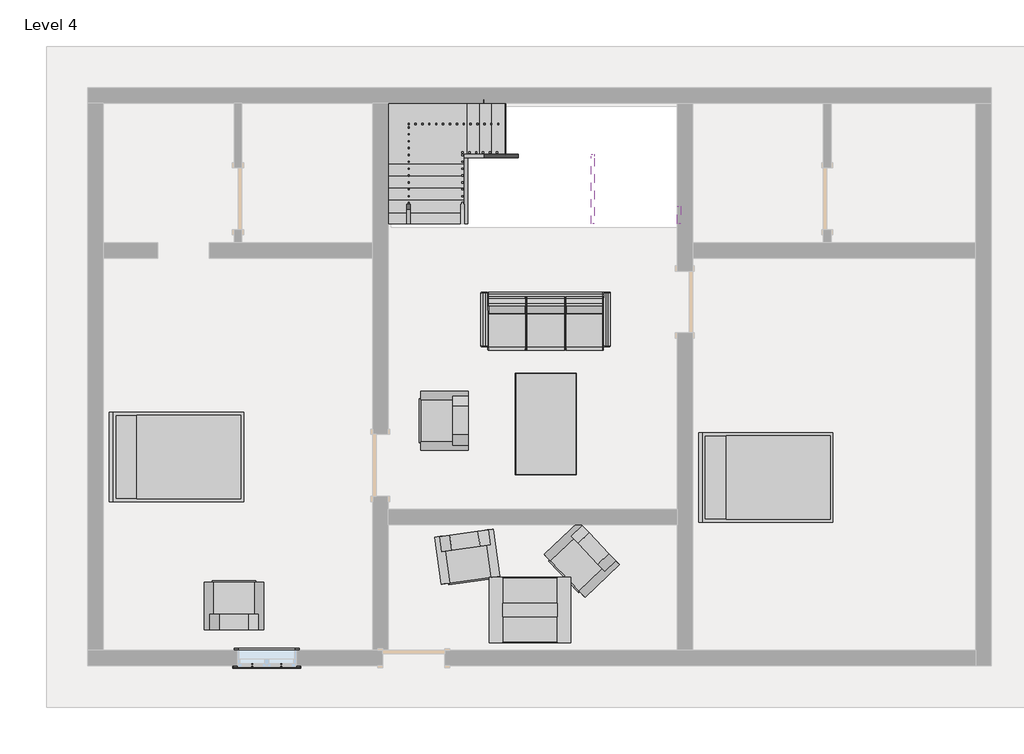
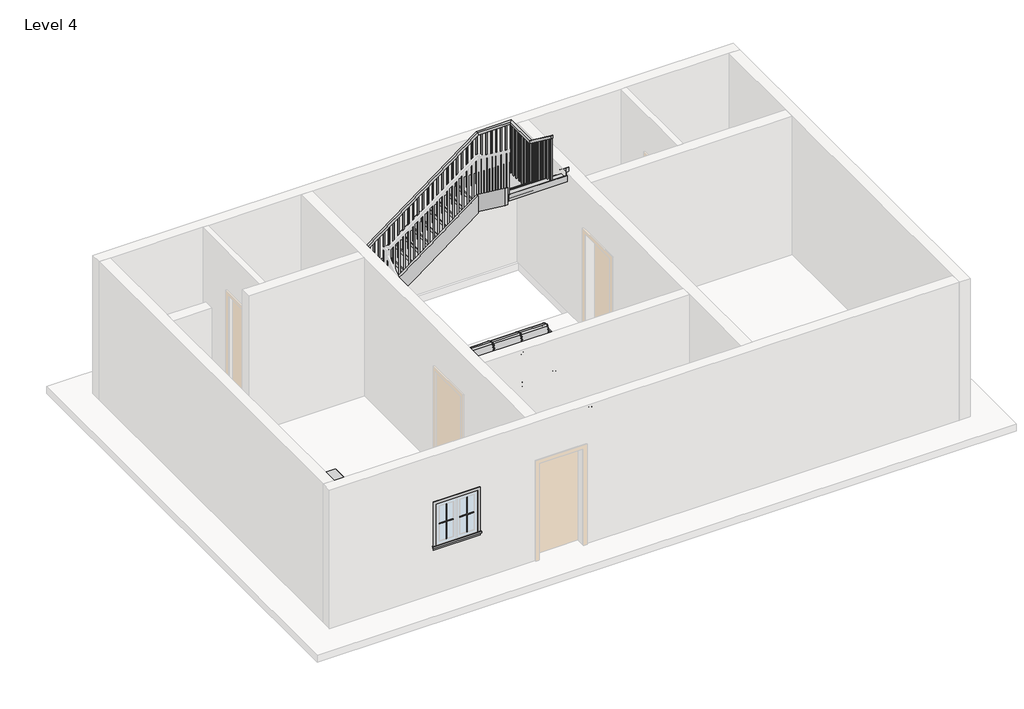
# One storey, part 2 of 2: 9 furniture elements, 6 members, 4 proxies, 1 railing, 1 stair flight.
"""IFC4 building model written with IfcOpenShell, lengths in millimetres."""

from ifc_helpers import new_model, si_unit, frame, origin, place, context, project, spatial, polyline, outline, extrude, faceted_brep, transform, mapped, element, save
from components import muntin_pattern_2x2_muntin_pattern_2x2_b3fe6957, muntin_pattern_2x2_muntin_pattern_2x2_3e0ecaf2, trim_window_exterior_flat_with_sill_41619996, trim_window_interior_flat_picture_frame_51c85655, furniture_2fc85b74, furniture_29a9adb8, furniture_57072a26, bed_17739_bed_17739_15c61121, chair_lounge_11461_couch_0866092f, dining_table_14755_dining_table_14755_d89cb775, wood_and_glass_coffee_table_17065_wood_and_glass_coffee_dbc724b2, stair_flight_3cceab32

model = new_model("IFC4")

# Units and contexts
model_context = context("Model", 3, world=origin())
ifc_project = project(units=[si_unit("LENGTHUNIT", "METRE", prefix="MILLI")], contexts=[model_context])

# Site, building, storey
site = spatial("IfcSite", under=ifc_project)
building = spatial("IfcBuilding", under=site)
storey = spatial("IfcBuildingStorey", under=building, Name="Level 4", Elevation=6400.8)

# Proxies
placement = place(None, origin())
muntin_pattern_2x2_muntin_pattern_2x2_shape = muntin_pattern_2x2_muntin_pattern_2x2_b3fe6957(model_context)
element("IfcBuildingElementProxy", 1, Name="Muntin Pattern_2x2 : Muntin Pattern_2x2", ObjectType="Muntin Pattern_2x2 : Muntin Pattern_2x2", at=placement, inside=storey, context=model_context, shape_type="MappedRepresentation", body=[
    mapped(muntin_pattern_2x2_muntin_pattern_2x2_shape, transform((-5069.3921642, -1799.3582394, 7537.7934313), x_axis=(-1.0, 0.0, 0.0), y_axis=(0.0, -1.0, 0.0), z_axis=(0.0, 0.0, 1.0))),
])
muntin_pattern_2x2_muntin_pattern_2x2_2_shape = muntin_pattern_2x2_muntin_pattern_2x2_3e0ecaf2(model_context)
element("IfcBuildingElementProxy", 2, Name="Muntin Pattern_2x2 : Muntin Pattern_2x2", ObjectType="Muntin Pattern_2x2 : Muntin Pattern_2x2", at=placement, inside=storey, context=model_context, shape_type="MappedRepresentation", body=[
    mapped(muntin_pattern_2x2_muntin_pattern_2x2_2_shape, transform((-5498.0171642, -1799.3582394, 7537.7934313), x_axis=(1.0, 0.0, 0.0), y_axis=(0.0, 1.0, 0.0), z_axis=(0.0, 0.0, 1.0))),
])
trim_window_exterior_flat_with_sill_shape = trim_window_exterior_flat_with_sill_41619996(model_context)
element("IfcBuildingElementProxy", 3, Name="Trim-Window-Exterior-Flat : with Sill", ObjectType="Trim-Window-Exterior-Flat : with Sill", at=placement, inside=storey, context=model_context, shape_type="MappedRepresentation", body=[
    mapped(trim_window_exterior_flat_with_sill_shape, transform((-5283.7046642, -1808.8832394, 8382.3434313), x_axis=(1.0, 0.0, 0.0), y_axis=(0.0, 0.0, 1.0), z_axis=(0.0, -1.0, 0.0))),
])
trim_window_interior_flat_picture_frame_shape = trim_window_interior_flat_picture_frame_51c85655(model_context)
element("IfcBuildingElementProxy", 4, Name="Trim-Window-Interior-Flat : Picture Frame", ObjectType="Trim-Window-Interior-Flat : Picture Frame", at=placement, inside=storey, context=model_context, shape_type="MappedRepresentation", body=[
    mapped(trim_window_interior_flat_picture_frame_shape, transform((-5283.7046642, -1580.2832394, 8382.3434313), x_axis=(-1.0, 0.0, 0.0), y_axis=(0.0, 0.0, 1.0), z_axis=(0.0, 1.0, 0.0))),
])

# Furniture
furniture_shape = furniture_2fc85b74(model_context)
furniture_2_shape = furniture_29a9adb8(model_context)
furniture_3_shape = furniture_57072a26(model_context)
element("IfcFurniture", 5, at=placement, inside=storey, context=model_context, shape_type="MappedRepresentation", body=[
    mapped(furniture_shape, transform((-1166.392994, 2905.4688314, 6400.8), x_axis=(1.0, 0.0, 0.0), y_axis=(0.0, 1.0, 0.0), z_axis=(0.0, 0.0, 1.0))),
    mapped(furniture_2_shape, transform((-1166.392994, 2905.4688314, 6400.8), x_axis=(1.0, 0.0, 0.0), y_axis=(0.0, 1.0, 0.0), z_axis=(0.0, 0.0, 1.0))),
    mapped(furniture_3_shape, transform((-1166.392994, 2905.4688314, 6400.8), x_axis=(1.0, 0.0, 0.0), y_axis=(0.0, 1.0, 0.0), z_axis=(0.0, 0.0, 1.0))),
])
bed_17739_bed_17739_shape = bed_17739_bed_17739_15c61121(model_context)
element("IfcFurniture", 6, ObjectType="Bed_17739 : Bed_17739", at=placement, inside=storey, context=model_context, shape_type="MappedRepresentation", body=[
    mapped(bed_17739_bed_17739_shape, transform((-6591.8046642, 1277.2167606, 6400.8), x_axis=(0.0, 1.0, 0.0), y_axis=(-1.0, 0.0, 0.0), z_axis=(0.0, 0.0, 1.0))),
])
element("IfcFurniture", 7, ObjectType="Bed_17739 : Bed_17739", at=placement, inside=storey, context=model_context, shape_type="MappedRepresentation", body=[
    mapped(bed_17739_bed_17739_shape, transform((2107.6953358, 972.4167606, 6400.8), x_axis=(0.0, 1.0, 0.0), y_axis=(-1.0, 0.0, 0.0), z_axis=(0.0, 0.0, 1.0))),
])
chair_lounge_11461_couch_shape = chair_lounge_11461_couch_0866092f(model_context)
element("IfcFurniture", 8, ObjectType="Chair-Lounge_11461 : Couch", at=placement, inside=storey, context=model_context, shape_type="MappedRepresentation", body=[
    mapped(chair_lounge_11461_couch_shape, transform((-5766.3046642, -1273.9095448, 6400.8), x_axis=(-1.0, 0.0, 0.0), y_axis=(0.0, -1.0, 0.0), z_axis=(0.0, 0.0, 1.0))),
])
element("IfcFurniture", 9, ObjectType="Chair-Lounge_11461 : Couch", at=placement, inside=storey, context=model_context, shape_type="MappedRepresentation", body=[
    mapped(chair_lounge_11461_couch_shape, transform((-2311.9046642, 1810.6167606, 6400.8), x_axis=(0.0, -1.0, 0.0), y_axis=(1.0, 0.0, 0.0), z_axis=(0.0, 0.0, 1.0))),
])
element("IfcFurniture", 10, ObjectType="Chair-Lounge_11461 : Couch", at=placement, inside=storey, context=model_context, shape_type="MappedRepresentation", body=[
    mapped(chair_lounge_11461_couch_shape, transform((-2372.9488995, 149.9169276, 6400.8), x_axis=(0.9905324493396854, 0.1372787922627668, 0.0), y_axis=(-0.1372787922627668, 0.9905324493396854, 0.0), z_axis=(0.0, 0.0, 1.0))),
])
element("IfcFurniture", 11, ObjectType="Chair-Lounge_11461 : Couch", at=placement, inside=storey, context=model_context, shape_type="MappedRepresentation", body=[
    mapped(chair_lounge_11461_couch_shape, transform((-378.7925234, 1.7617886, 6400.8), x_axis=(0.6894995564131732, -0.7242861048688133, 0.0), y_axis=(0.7242861048688133, 0.6894995564131732, 0.0), z_axis=(0.0, 0.0, 1.0))),
])
dining_table_14755_dining_table_14755_shape = dining_table_14755_dining_table_14755_d89cb775(model_context)
element("IfcFurniture", 12, ObjectType="Dining_table_14755 : Dining_table_14755", at=placement, inside=storey, context=model_context, shape_type="MappedRepresentation", body=[
    mapped(dining_table_14755_dining_table_14755_shape, transform((-711.7046642, 1010.5167606, 6400.8), x_axis=(0.0, 1.0, 0.0), y_axis=(-1.0, 0.0, 0.0), z_axis=(0.0, 0.0, 1.0))),
])
wood_and_glass_coffee_table_17065_wood_and_glass_coffee_shape = wood_and_glass_coffee_table_17065_wood_and_glass_coffee_dbc724b2(model_context)
element("IfcFurniture", 13, ObjectType="Wood_and_Glass_Coffee_Table_17065 : Wood_and_Glass_Coffee_Table_17065", at=placement, inside=storey, context=model_context, shape_type="MappedRepresentation", body=[
    mapped(wood_and_glass_coffee_table_17065_wood_and_glass_coffee_shape, transform((-1397.5046642, -983.3832394, 6400.8), x_axis=(1.0, 0.0, 0.0), y_axis=(0.0, 1.0, 0.0), z_axis=(0.0, 0.0, 1.0))),
])

# Members
element("IfcMember", 14, ObjectType="Stringer - 2\" Width", at=placement, inside=storey, context=model_context, shape_type="SweptSolid", body=[
    extrude(outline(polyline([(4718.9167606, 6400.8), (4718.9167606, 6548.4508226), (5113.281957, 6548.4508226), (4911.6463024, 6400.8), (4718.9167606, 6400.8)])), frame((-3543.8046642, 0.0, 0.0), z_axis=(1.0, 0.0, 0.0), x_axis=(0.0, 1.0, 0.0)), (0.0, 0.0, 1.0), 50.8),
])
element("IfcMember", 15, ObjectType="Stringer - 2\" Width", at=placement, inside=storey, context=model_context, shape_type="SweptSolid", body=[
    extrude(outline(polyline([(7561.6387795, -1623.6098785), (8217.5484291, -743.5977653), (8217.5484291, -1253.6320422), (7561.6387795, -2133.6441554), (7561.6387795, -1623.6098785)])), frame((0.0, 6496.9167606, 0.0), z_axis=(0.0, 1.0, 0.0), x_axis=(0.0, 0.0, 1.0)), (0.0, 0.0, 1.0), 50.8),
])
element("IfcMember", 16, ObjectType="Stringer - 2\" Width", at=placement, inside=storey, context=model_context, shape_type="SweptSolid", body=[
    extrude(outline(polyline([(4718.9167606, 9348.8227901), (4718.9167606, 9542.7652405), (4979.1229954, 9348.8227901), (4718.9167606, 9348.8227901)])), frame((774.1953358, 0.0, 0.0), z_axis=(1.0, 0.0, 0.0), x_axis=(0.0, 1.0, 0.0)), (0.0, 0.0, 1.0), 50.8),
])
element("IfcMember", 17, ObjectType="Stringer - 2\" Width", at=placement, inside=storey, context=model_context, shape_type="SweptSolid", body=[
    extrude(outline(polyline([(4718.9167606, 6400.8), (4718.9167606, 6637.4522719), (5695.7536537, 7352.7561753), (5695.7536537, 6974.9747195), (4911.6463024, 6400.8), (4718.9167606, 6400.8)])), frame((-2368.6972892, 0.0, 0.0), z_axis=(1.0, 0.0, 0.0), x_axis=(0.0, 1.0, 0.0)), (0.0, 0.0, 1.0), 50.8),
])
element("IfcMember", 18, ObjectType="Stringer - 2\" Width", at=placement, inside=storey, context=model_context, shape_type="SweptSolid", body=[
    extrude(outline(polyline([(7386.4438971, -2368.6972892), (7012.1738041, -2368.6972892), (7012.1738041, -2360.8087204), (8402.2389392, -495.8046642), (8776.8250342, -495.8046642), (8776.8250342, -503.2692636), (7386.4438971, -2368.6972892)])), frame((0.0, 5695.7536537, 0.0), z_axis=(0.0, 1.0, 0.0), x_axis=(0.0, 0.0, 1.0)), (0.0, 0.0, 1.0), 50.8),
])
element("IfcMember", 19, ObjectType="Stringer - 2\" Width", at=placement, inside=storey, context=model_context, shape_type="SweptSolid", body=[
    extrude(outline(polyline([(5746.5536537, 8776.8250342), (5746.5536537, 8440.1022932), (5688.2891085, 8440.1022932), (4718.9167606, 9162.6155283), (4718.9167606, 9542.7652405), (5746.5536537, 8776.8250342)])), frame((-495.8046642, 0.0, 0.0), z_axis=(1.0, 0.0, 0.0), x_axis=(0.0, 1.0, 0.0)), (0.0, 0.0, 1.0), 50.8),
])

# Railing
element("IfcRailing", 20, ObjectType="Handrail - Rectangular", at=placement, inside=storey, context=model_context, shape_type="SolidModel", body=[
    faceted_brep([(-3213.6046642, 4718.9167606, 7447.7217391), (-3213.6046642, 4718.9167606, 7384.3634439), (-3162.8046642, 4718.9167606, 7384.3634439), (-3162.8046642, 4718.9167606, 7447.7217391), (-3213.6046642, 5555.0306195, 8070.912193), (-3213.6046642, 5571.8796657, 8020.112193), (-3162.8046642, 5571.8796657, 8020.112193), (-3162.8046642, 5555.0306195, 8070.912193), (-3213.6046642, 6217.5167606, 8070.912193), (-3213.6046642, 6217.5167606, 8020.112193), (-3162.8046642, 6166.7167606, 8020.112193), (-3162.8046642, 6166.7167606, 8070.912193), (-2551.1185231, 6217.5167606, 8070.912193), (-2534.269477, 6217.5167606, 8020.112193), (-2534.269477, 6166.7167606, 8020.112193), (-2551.1185231, 6166.7167606, 8070.912193), (-239.7185231, 6217.5167606, 9793.6948017), (-222.869477, 6217.5167606, 9742.8948017), (-222.869477, 6166.7167606, 9742.8948017), (-239.7185231, 6166.7167606, 9793.6948017), (494.7953358, 6217.5167606, 9793.6948017), (494.7953358, 6217.5167606, 9742.8948017), (443.9953358, 6166.7167606, 9742.8948017), (443.9953358, 6166.7167606, 9793.6948017), (494.7953358, 5483.0029017, 9793.6948017), (494.7953358, 5466.1538556, 9742.8948017), (443.9953358, 5466.1538556, 9742.8948017), (443.9953358, 5483.0029017, 9793.6948017), (494.7953358, 4718.9167606, 10363.2), (443.9953358, 4718.9167606, 10363.2), (443.9953358, 4718.9167606, 10299.8417047), (494.7953358, 4718.9167606, 10299.8417047)], [[[0, 1, 2, 3]], [[1, 0, 4, 5]], [[2, 1, 5, 6]], [[3, 2, 6, 7]], [[0, 3, 7, 4]], [[5, 4, 8, 9]], [[6, 5, 9, 10]], [[7, 6, 10, 11]], [[4, 7, 11, 8]], [[9, 8, 12, 13]], [[10, 9, 13, 14]], [[11, 10, 14, 15]], [[8, 11, 15, 12]], [[13, 12, 16, 17]], [[14, 13, 17, 18]], [[15, 14, 18, 19]], [[12, 15, 19, 16]], [[17, 16, 20, 21]], [[18, 17, 21, 22]], [[19, 18, 22, 23]], [[16, 19, 23, 20]], [[21, 20, 24, 25]], [[22, 21, 25, 26]], [[23, 22, 26, 27]], [[20, 23, 27, 24]], [[28, 29, 30, 31]], [[25, 24, 28, 31]], [[26, 25, 31, 30]], [[27, 26, 30, 29]], [[24, 27, 29, 28]]]),
    extrude(outline(polyline([(4779.2417606, 10254.8789718), (4779.2417606, 9316.2782609), (4760.1917606, 9316.2782609), (4760.1917606, 10269.0777296), (4779.2417606, 10254.8789718)])), frame((459.8703358, 0.0, 0.0), z_axis=(1.0, 0.0, 0.0), x_axis=(0.0, 1.0, 0.0)), (0.0, 0.0, 1.0), 19.05),
    extrude(outline(polyline([(4880.8417606, 10179.1522637), (4880.8417606, 9316.2782609), (4861.7917606, 9316.2782609), (4861.7917606, 10193.3510215), (4880.8417606, 10179.1522637)])), frame((459.8703358, 0.0, 0.0), z_axis=(1.0, 0.0, 0.0), x_axis=(0.0, 1.0, 0.0)), (0.0, 0.0, 1.0), 19.05),
    extrude(outline(polyline([(4982.4417606, 10103.4255557), (4982.4417606, 9183.7565217), (4963.3917606, 9183.7565217), (4963.3917606, 10117.6243134), (4982.4417606, 10103.4255557)])), frame((459.8703358, 0.0, 0.0), z_axis=(1.0, 0.0, 0.0), x_axis=(0.0, 1.0, 0.0)), (0.0, 0.0, 1.0), 19.05),
    extrude(outline(polyline([(5084.0417606, 10027.6988476), (5084.0417606, 9183.7565217), (5064.9917606, 9183.7565217), (5064.9917606, 10041.8976054), (5084.0417606, 10027.6988476)])), frame((459.8703358, 0.0, 0.0), z_axis=(1.0, 0.0, 0.0), x_axis=(0.0, 1.0, 0.0)), (0.0, 0.0, 1.0), 19.05),
    extrude(outline(polyline([(5185.6417606, 9951.9721395), (5185.6417606, 9051.2347826), (5166.5917606, 9051.2347826), (5166.5917606, 9966.1708973), (5185.6417606, 9951.9721395)])), frame((459.8703358, 0.0, 0.0), z_axis=(1.0, 0.0, 0.0), x_axis=(0.0, 1.0, 0.0)), (0.0, 0.0, 1.0), 19.05),
    extrude(outline(polyline([(5287.2417606, 9876.2454314), (5287.2417606, 8918.7130435), (5268.1917606, 8918.7130435), (5268.1917606, 9890.4441892), (5287.2417606, 9876.2454314)])), frame((459.8703358, 0.0, 0.0), z_axis=(1.0, 0.0, 0.0), x_axis=(0.0, 1.0, 0.0)), (0.0, 0.0, 1.0), 19.05),
    extrude(outline(polyline([(5388.8417606, 9800.5187234), (5388.8417606, 8918.7130435), (5369.7917606, 8918.7130435), (5369.7917606, 9814.7174811), (5388.8417606, 9800.5187234)])), frame((459.8703358, 0.0, 0.0), z_axis=(1.0, 0.0, 0.0), x_axis=(0.0, 1.0, 0.0)), (0.0, 0.0, 1.0), 19.05),
    extrude(outline(polyline([(5490.4417606, 9724.7920153), (5490.4417606, 8786.1913043), (5471.3917606, 8786.1913043), (5471.3917606, 9738.9907731), (5490.4417606, 9724.7920153)])), frame((459.8703358, 0.0, 0.0), z_axis=(1.0, 0.0, 0.0), x_axis=(0.0, 1.0, 0.0)), (0.0, 0.0, 1.0), 19.05),
    extrude(outline(polyline([(478.9203358, 5592.0417606), (478.9203358, 5572.9917606), (459.8703358, 5572.9917606), (459.8703358, 5592.0417606), (478.9203358, 5592.0417606)])), frame((0.0, 0.0, 8786.1913043), z_axis=(0.0, 0.0, 1.0), x_axis=(1.0, 0.0, 0.0)), (0.0, 0.0, 1.0), 956.7034973),
    extrude(outline(polyline([(478.9203358, 5693.6417606), (478.9203358, 5674.5917606), (459.8703358, 5674.5917606), (459.8703358, 5693.6417606), (478.9203358, 5693.6417606)])), frame((0.0, 0.0, 8653.6695652), z_axis=(0.0, 0.0, 1.0), x_axis=(1.0, 0.0, 0.0)), (0.0, 0.0, 1.0), 1089.2252364),
    extrude(outline(polyline([(478.9203358, 5795.2417606), (478.9203358, 5776.1917606), (459.8703358, 5776.1917606), (459.8703358, 5795.2417606), (478.9203358, 5795.2417606)])), frame((0.0, 0.0, 8653.6695652), z_axis=(0.0, 0.0, 1.0), x_axis=(1.0, 0.0, 0.0)), (0.0, 0.0, 1.0), 1089.2252364),
    extrude(outline(polyline([(478.9203358, 5896.8417606), (478.9203358, 5877.7917606), (459.8703358, 5877.7917606), (459.8703358, 5896.8417606), (478.9203358, 5896.8417606)])), frame((0.0, 0.0, 8653.6695652), z_axis=(0.0, 0.0, 1.0), x_axis=(1.0, 0.0, 0.0)), (0.0, 0.0, 1.0), 1089.2252364),
    extrude(outline(polyline([(478.9203358, 5998.4417606), (478.9203358, 5979.3917606), (459.8703358, 5979.3917606), (459.8703358, 5998.4417606), (478.9203358, 5998.4417606)])), frame((0.0, 0.0, 8653.6695652), z_axis=(0.0, 0.0, 1.0), x_axis=(1.0, 0.0, 0.0)), (0.0, 0.0, 1.0), 1089.2252364),
    extrude(outline(polyline([(478.9203358, 6100.0417606), (478.9203358, 6080.9917606), (459.8703358, 6080.9917606), (459.8703358, 6100.0417606), (478.9203358, 6100.0417606)])), frame((0.0, 0.0, 8653.6695652), z_axis=(0.0, 0.0, 1.0), x_axis=(1.0, 0.0, 0.0)), (0.0, 0.0, 1.0), 1089.2252364),
    extrude(outline(polyline([(358.2703358, 6201.6417606), (377.3203358, 6201.6417606), (377.3203358, 6182.5917606), (358.2703358, 6182.5917606), (358.2703358, 6201.6417606)])), frame((0.0, 0.0, 8653.6695652), z_axis=(0.0, 0.0, 1.0), x_axis=(1.0, 0.0, 0.0)), (0.0, 0.0, 1.0), 1089.2252364),
    extrude(outline(polyline([(256.6703358, 6201.6417606), (275.7203358, 6201.6417606), (275.7203358, 6182.5917606), (256.6703358, 6182.5917606), (256.6703358, 6201.6417606)])), frame((0.0, 0.0, 8653.6695652), z_axis=(0.0, 0.0, 1.0), x_axis=(1.0, 0.0, 0.0)), (0.0, 0.0, 1.0), 1089.2252364),
    extrude(outline(polyline([(155.0703358, 6201.6417606), (174.1203358, 6201.6417606), (174.1203358, 6182.5917606), (155.0703358, 6182.5917606), (155.0703358, 6201.6417606)])), frame((0.0, 0.0, 8653.6695652), z_axis=(0.0, 0.0, 1.0), x_axis=(1.0, 0.0, 0.0)), (0.0, 0.0, 1.0), 1089.2252364),
    extrude(outline(polyline([(53.4703358, 6201.6417606), (72.5203358, 6201.6417606), (72.5203358, 6182.5917606), (53.4703358, 6182.5917606), (53.4703358, 6201.6417606)])), frame((0.0, 0.0, 8653.6695652), z_axis=(0.0, 0.0, 1.0), x_axis=(1.0, 0.0, 0.0)), (0.0, 0.0, 1.0), 1089.2252364),
    extrude(outline(polyline([(-48.1296642, 6201.6417606), (-29.0796642, 6201.6417606), (-29.0796642, 6182.5917606), (-48.1296642, 6182.5917606), (-48.1296642, 6201.6417606)])), frame((0.0, 0.0, 8653.6695652), z_axis=(0.0, 0.0, 1.0), x_axis=(1.0, 0.0, 0.0)), (0.0, 0.0, 1.0), 1089.2252364),
    extrude(outline(polyline([(-149.7296642, 6201.6417606), (-130.6796642, 6201.6417606), (-130.6796642, 6182.5917606), (-149.7296642, 6182.5917606), (-149.7296642, 6201.6417606)])), frame((0.0, 0.0, 8653.6695652), z_axis=(0.0, 0.0, 1.0), x_axis=(1.0, 0.0, 0.0)), (0.0, 0.0, 1.0), 1089.2252364),
    extrude(outline(polyline([(9721.6822397, -251.3296642), (8653.6695652, -251.3296642), (8653.6695652, -232.2796642), (9735.8809975, -232.2796642), (9721.6822397, -251.3296642)])), frame((0.0, 6182.5917606, 0.0), z_axis=(0.0, 1.0, 0.0), x_axis=(0.0, 0.0, 1.0)), (0.0, 0.0, 1.0), 19.05),
    extrude(outline(polyline([(9645.9555316, -352.9296642), (8653.6695652, -352.9296642), (8653.6695652, -333.8796642), (9660.1542894, -333.8796642), (9645.9555316, -352.9296642)])), frame((0.0, 6182.5917606, 0.0), z_axis=(0.0, 1.0, 0.0), x_axis=(0.0, 0.0, 1.0)), (0.0, 0.0, 1.0), 19.05),
    extrude(outline(polyline([(9570.2288236, -454.5296642), (8653.6695652, -454.5296642), (8653.6695652, -435.4796642), (9584.4275813, -435.4796642), (9570.2288236, -454.5296642)])), frame((0.0, 6182.5917606, 0.0), z_axis=(0.0, 1.0, 0.0), x_axis=(0.0, 0.0, 1.0)), (0.0, 0.0, 1.0), 19.05),
    extrude(outline(polyline([(9494.5021155, -556.1296642), (8521.1478261, -556.1296642), (8521.1478261, -537.0796642), (9508.7008733, -537.0796642), (9494.5021155, -556.1296642)])), frame((0.0, 6182.5917606, 0.0), z_axis=(0.0, 1.0, 0.0), x_axis=(0.0, 0.0, 1.0)), (0.0, 0.0, 1.0), 19.05),
    extrude(outline(polyline([(9418.7754074, -657.7296642), (8521.1478261, -657.7296642), (8521.1478261, -638.6796642), (9432.9741652, -638.6796642), (9418.7754074, -657.7296642)])), frame((0.0, 6182.5917606, 0.0), z_axis=(0.0, 1.0, 0.0), x_axis=(0.0, 0.0, 1.0)), (0.0, 0.0, 1.0), 19.05),
    extrude(outline(polyline([(9343.0486993, -759.3296642), (8388.626087, -759.3296642), (8388.626087, -740.2796642), (9357.2474571, -740.2796642), (9343.0486993, -759.3296642)])), frame((0.0, 6182.5917606, 0.0), z_axis=(0.0, 1.0, 0.0), x_axis=(0.0, 0.0, 1.0)), (0.0, 0.0, 1.0), 19.05),
    extrude(outline(polyline([(9267.3219913, -860.9296642), (8388.626087, -860.9296642), (8388.626087, -841.8796642), (9281.520749, -841.8796642), (9267.3219913, -860.9296642)])), frame((0.0, 6182.5917606, 0.0), z_axis=(0.0, 1.0, 0.0), x_axis=(0.0, 0.0, 1.0)), (0.0, 0.0, 1.0), 19.05),
    extrude(outline(polyline([(9191.5952832, -962.5296642), (8256.1043478, -962.5296642), (8256.1043478, -943.4796642), (9205.794041, -943.4796642), (9191.5952832, -962.5296642)])), frame((0.0, 6182.5917606, 0.0), z_axis=(0.0, 1.0, 0.0), x_axis=(0.0, 0.0, 1.0)), (0.0, 0.0, 1.0), 19.05),
    extrude(outline(polyline([(9115.8685751, -1064.1296642), (8256.1043478, -1064.1296642), (8256.1043478, -1045.0796642), (9130.0673329, -1045.0796642), (9115.8685751, -1064.1296642)])), frame((0.0, 6182.5917606, 0.0), z_axis=(0.0, 1.0, 0.0), x_axis=(0.0, 0.0, 1.0)), (0.0, 0.0, 1.0), 19.05),
    extrude(outline(polyline([(9040.141867, -1165.7296642), (8123.5826087, -1165.7296642), (8123.5826087, -1146.6796642), (9054.3406248, -1146.6796642), (9040.141867, -1165.7296642)])), frame((0.0, 6182.5917606, 0.0), z_axis=(0.0, 1.0, 0.0), x_axis=(0.0, 0.0, 1.0)), (0.0, 0.0, 1.0), 19.05),
    extrude(outline(polyline([(8964.415159, -1267.3296642), (7991.0608696, -1267.3296642), (7991.0608696, -1248.2796642), (8978.6139167, -1248.2796642), (8964.415159, -1267.3296642)])), frame((0.0, 6182.5917606, 0.0), z_axis=(0.0, 1.0, 0.0), x_axis=(0.0, 0.0, 1.0)), (0.0, 0.0, 1.0), 19.05),
    extrude(outline(polyline([(8888.6884509, -1368.9296642), (7991.0608696, -1368.9296642), (7991.0608696, -1349.8796642), (8902.8872087, -1349.8796642), (8888.6884509, -1368.9296642)])), frame((0.0, 6182.5917606, 0.0), z_axis=(0.0, 1.0, 0.0), x_axis=(0.0, 0.0, 1.0)), (0.0, 0.0, 1.0), 19.05),
    extrude(outline(polyline([(8812.9617428, -1470.5296642), (7858.5391304, -1470.5296642), (7858.5391304, -1451.4796642), (8827.1605006, -1451.4796642), (8812.9617428, -1470.5296642)])), frame((0.0, 6182.5917606, 0.0), z_axis=(0.0, 1.0, 0.0), x_axis=(0.0, 0.0, 1.0)), (0.0, 0.0, 1.0), 19.05),
    extrude(outline(polyline([(8737.2350347, -1572.1296642), (7858.5391304, -1572.1296642), (7858.5391304, -1553.0796642), (8751.4337925, -1553.0796642), (8737.2350347, -1572.1296642)])), frame((0.0, 6182.5917606, 0.0), z_axis=(0.0, 1.0, 0.0), x_axis=(0.0, 0.0, 1.0)), (0.0, 0.0, 1.0), 19.05),
    extrude(outline(polyline([(8661.5083267, -1673.7296642), (7726.0173913, -1673.7296642), (7726.0173913, -1654.6796642), (8675.7070844, -1654.6796642), (8661.5083267, -1673.7296642)])), frame((0.0, 6182.5917606, 0.0), z_axis=(0.0, 1.0, 0.0), x_axis=(0.0, 0.0, 1.0)), (0.0, 0.0, 1.0), 19.05),
    extrude(outline(polyline([(8585.7816186, -1775.3296642), (7726.0173913, -1775.3296642), (7726.0173913, -1756.2796642), (8599.9803764, -1756.2796642), (8585.7816186, -1775.3296642)])), frame((0.0, 6182.5917606, 0.0), z_axis=(0.0, 1.0, 0.0), x_axis=(0.0, 0.0, 1.0)), (0.0, 0.0, 1.0), 19.05),
    extrude(outline(polyline([(8510.0549105, -1876.9296642), (7593.4956522, -1876.9296642), (7593.4956522, -1857.8796642), (8524.2536683, -1857.8796642), (8510.0549105, -1876.9296642)])), frame((0.0, 6182.5917606, 0.0), z_axis=(0.0, 1.0, 0.0), x_axis=(0.0, 0.0, 1.0)), (0.0, 0.0, 1.0), 19.05),
    extrude(outline(polyline([(8434.3282025, -1978.5296642), (7460.973913, -1978.5296642), (7460.973913, -1959.4796642), (8448.5269602, -1959.4796642), (8434.3282025, -1978.5296642)])), frame((0.0, 6182.5917606, 0.0), z_axis=(0.0, 1.0, 0.0), x_axis=(0.0, 0.0, 1.0)), (0.0, 0.0, 1.0), 19.05),
    extrude(outline(polyline([(8358.6014944, -2080.1296642), (7460.973913, -2080.1296642), (7460.973913, -2061.0796642), (8372.8002521, -2061.0796642), (8358.6014944, -2080.1296642)])), frame((0.0, 6182.5917606, 0.0), z_axis=(0.0, 1.0, 0.0), x_axis=(0.0, 0.0, 1.0)), (0.0, 0.0, 1.0), 19.05),
    extrude(outline(polyline([(8282.8747863, -2181.7296642), (7328.4521739, -2181.7296642), (7328.4521739, -2162.6796642), (8297.0735441, -2162.6796642), (8282.8747863, -2181.7296642)])), frame((0.0, 6182.5917606, 0.0), z_axis=(0.0, 1.0, 0.0), x_axis=(0.0, 0.0, 1.0)), (0.0, 0.0, 1.0), 19.05),
    extrude(outline(polyline([(8207.1480782, -2283.3296642), (7328.4521739, -2283.3296642), (7328.4521739, -2264.2796642), (8221.346836, -2264.2796642), (8207.1480782, -2283.3296642)])), frame((0.0, 6182.5917606, 0.0), z_axis=(0.0, 1.0, 0.0), x_axis=(0.0, 0.0, 1.0)), (0.0, 0.0, 1.0), 19.05),
    extrude(outline(polyline([(8131.4213702, -2384.9296642), (7195.9304348, -2384.9296642), (7195.9304348, -2365.8796642), (8145.6201279, -2365.8796642), (8131.4213702, -2384.9296642)])), frame((0.0, 6182.5917606, 0.0), z_axis=(0.0, 1.0, 0.0), x_axis=(0.0, 0.0, 1.0)), (0.0, 0.0, 1.0), 19.05),
    extrude(outline(polyline([(8055.6946621, -2486.5296642), (7195.9304348, -2486.5296642), (7195.9304348, -2467.4796642), (8069.8934198, -2467.4796642), (8055.6946621, -2486.5296642)])), frame((0.0, 6182.5917606, 0.0), z_axis=(0.0, 1.0, 0.0), x_axis=(0.0, 0.0, 1.0)), (0.0, 0.0, 1.0), 19.05),
    extrude(outline(polyline([(-2588.1296642, 6201.6417606), (-2569.0796642, 6201.6417606), (-2569.0796642, 6182.5917606), (-2588.1296642, 6182.5917606), (-2588.1296642, 6201.6417606)])), frame((0.0, 0.0, 7195.9304348), z_axis=(0.0, 0.0, 1.0), x_axis=(1.0, 0.0, 0.0)), (0.0, 0.0, 1.0), 824.1817582),
    extrude(outline(polyline([(-2689.7296642, 6201.6417606), (-2670.6796642, 6201.6417606), (-2670.6796642, 6182.5917606), (-2689.7296642, 6182.5917606), (-2689.7296642, 6201.6417606)])), frame((0.0, 0.0, 7195.9304348), z_axis=(0.0, 0.0, 1.0), x_axis=(1.0, 0.0, 0.0)), (0.0, 0.0, 1.0), 824.1817582),
    extrude(outline(polyline([(-2791.3296642, 6201.6417606), (-2772.2796642, 6201.6417606), (-2772.2796642, 6182.5917606), (-2791.3296642, 6182.5917606), (-2791.3296642, 6201.6417606)])), frame((0.0, 0.0, 7195.9304348), z_axis=(0.0, 0.0, 1.0), x_axis=(1.0, 0.0, 0.0)), (0.0, 0.0, 1.0), 824.1817582),
    extrude(outline(polyline([(-2892.9296642, 6201.6417606), (-2873.8796642, 6201.6417606), (-2873.8796642, 6182.5917606), (-2892.9296642, 6182.5917606), (-2892.9296642, 6201.6417606)])), frame((0.0, 0.0, 7195.9304348), z_axis=(0.0, 0.0, 1.0), x_axis=(1.0, 0.0, 0.0)), (0.0, 0.0, 1.0), 824.1817582),
    extrude(outline(polyline([(-2994.5296642, 6201.6417606), (-2975.4796642, 6201.6417606), (-2975.4796642, 6182.5917606), (-2994.5296642, 6182.5917606), (-2994.5296642, 6201.6417606)])), frame((0.0, 0.0, 7195.9304348), z_axis=(0.0, 0.0, 1.0), x_axis=(1.0, 0.0, 0.0)), (0.0, 0.0, 1.0), 824.1817582),
    extrude(outline(polyline([(-3096.1296642, 6201.6417606), (-3077.0796642, 6201.6417606), (-3077.0796642, 6182.5917606), (-3096.1296642, 6182.5917606), (-3096.1296642, 6201.6417606)])), frame((0.0, 0.0, 7195.9304348), z_axis=(0.0, 0.0, 1.0), x_axis=(1.0, 0.0, 0.0)), (0.0, 0.0, 1.0), 824.1817582),
    extrude(outline(polyline([(-3197.7296642, 6131.7917606), (-3197.7296642, 6150.8417606), (-3178.6796642, 6150.8417606), (-3178.6796642, 6131.7917606), (-3197.7296642, 6131.7917606)])), frame((0.0, 0.0, 7195.9304348), z_axis=(0.0, 0.0, 1.0), x_axis=(1.0, 0.0, 0.0)), (0.0, 0.0, 1.0), 824.1817582),
    extrude(outline(polyline([(-3197.7296642, 6030.1917606), (-3197.7296642, 6049.2417606), (-3178.6796642, 6049.2417606), (-3178.6796642, 6030.1917606), (-3197.7296642, 6030.1917606)])), frame((0.0, 0.0, 7195.9304348), z_axis=(0.0, 0.0, 1.0), x_axis=(1.0, 0.0, 0.0)), (0.0, 0.0, 1.0), 824.1817582),
    extrude(outline(polyline([(-3197.7296642, 5928.5917606), (-3197.7296642, 5947.6417606), (-3178.6796642, 5947.6417606), (-3178.6796642, 5928.5917606), (-3197.7296642, 5928.5917606)])), frame((0.0, 0.0, 7195.9304348), z_axis=(0.0, 0.0, 1.0), x_axis=(1.0, 0.0, 0.0)), (0.0, 0.0, 1.0), 824.1817582),
    extrude(outline(polyline([(-3197.7296642, 5826.9917606), (-3197.7296642, 5846.0417606), (-3178.6796642, 5846.0417606), (-3178.6796642, 5826.9917606), (-3197.7296642, 5826.9917606)])), frame((0.0, 0.0, 7195.9304348), z_axis=(0.0, 0.0, 1.0), x_axis=(1.0, 0.0, 0.0)), (0.0, 0.0, 1.0), 824.1817582),
    extrude(outline(polyline([(-3197.7296642, 5725.3917606), (-3197.7296642, 5744.4417606), (-3178.6796642, 5744.4417606), (-3178.6796642, 5725.3917606), (-3197.7296642, 5725.3917606)])), frame((0.0, 0.0, 7195.9304348), z_axis=(0.0, 0.0, 1.0), x_axis=(1.0, 0.0, 0.0)), (0.0, 0.0, 1.0), 824.1817582),
    extrude(outline(polyline([(-3197.7296642, 5623.7917606), (-3197.7296642, 5642.8417606), (-3178.6796642, 5642.8417606), (-3178.6796642, 5623.7917606), (-3197.7296642, 5623.7917606)])), frame((0.0, 0.0, 7195.9304348), z_axis=(0.0, 0.0, 1.0), x_axis=(1.0, 0.0, 0.0)), (0.0, 0.0, 1.0), 824.1817582),
    extrude(outline(polyline([(5541.2417606, 7997.2764873), (5541.2417606, 7063.4086957), (5522.1917606, 7063.4086957), (5522.1917606, 7983.0777296), (5541.2417606, 7997.2764873)])), frame((-3197.7296642, 0.0, 0.0), z_axis=(1.0, 0.0, 0.0), x_axis=(0.0, 1.0, 0.0)), (0.0, 0.0, 1.0), 19.05),
    extrude(outline(polyline([(5439.6417606, 7921.5497793), (5439.6417606, 7063.4086957), (5420.5917606, 7063.4086957), (5420.5917606, 7907.3510215), (5439.6417606, 7921.5497793)])), frame((-3197.7296642, 0.0, 0.0), z_axis=(1.0, 0.0, 0.0), x_axis=(0.0, 1.0, 0.0)), (0.0, 0.0, 1.0), 19.05),
    extrude(outline(polyline([(5338.0417606, 7845.8230712), (5338.0417606, 6930.8869565), (5318.9917606, 6930.8869565), (5318.9917606, 7831.6243134), (5338.0417606, 7845.8230712)])), frame((-3197.7296642, 0.0, 0.0), z_axis=(1.0, 0.0, 0.0), x_axis=(0.0, 1.0, 0.0)), (0.0, 0.0, 1.0), 19.05),
    extrude(outline(polyline([(5236.4417606, 7770.0963631), (5236.4417606, 6798.3652174), (5217.3917606, 6798.3652174), (5217.3917606, 7755.8976054), (5236.4417606, 7770.0963631)])), frame((-3197.7296642, 0.0, 0.0), z_axis=(1.0, 0.0, 0.0), x_axis=(0.0, 1.0, 0.0)), (0.0, 0.0, 1.0), 19.05),
    extrude(outline(polyline([(5134.8417606, 7694.369655), (5134.8417606, 6798.3652174), (5115.7917606, 6798.3652174), (5115.7917606, 7680.1708973), (5134.8417606, 7694.369655)])), frame((-3197.7296642, 0.0, 0.0), z_axis=(1.0, 0.0, 0.0), x_axis=(0.0, 1.0, 0.0)), (0.0, 0.0, 1.0), 19.05),
    extrude(outline(polyline([(5033.2417606, 7618.642947), (5033.2417606, 6665.8434783), (5014.1917606, 6665.8434783), (5014.1917606, 7604.4441892), (5033.2417606, 7618.642947)])), frame((-3197.7296642, 0.0, 0.0), z_axis=(1.0, 0.0, 0.0), x_axis=(0.0, 1.0, 0.0)), (0.0, 0.0, 1.0), 19.05),
    extrude(outline(polyline([(4931.6417606, 7542.9162389), (4931.6417606, 6665.8434783), (4912.5917606, 6665.8434783), (4912.5917606, 7528.7174811), (4931.6417606, 7542.9162389)])), frame((-3197.7296642, 0.0, 0.0), z_axis=(1.0, 0.0, 0.0), x_axis=(0.0, 1.0, 0.0)), (0.0, 0.0, 1.0), 19.05),
    extrude(outline(polyline([(4830.0417606, 7467.1895308), (4830.0417606, 6533.3217391), (4810.9917606, 6533.3217391), (4810.9917606, 7452.9907731), (4830.0417606, 7467.1895308)])), frame((-3197.7296642, 0.0, 0.0), z_axis=(1.0, 0.0, 0.0), x_axis=(0.0, 1.0, 0.0)), (0.0, 0.0, 1.0), 19.05),
    extrude(outline(polyline([(459.8703358, 6201.6417606), (478.9203358, 6201.6417606), (478.9203358, 6182.5917606), (459.8703358, 6182.5917606), (459.8703358, 6201.6417606)])), frame((0.0, 0.0, 8653.6695652), z_axis=(0.0, 0.0, 1.0), x_axis=(1.0, 0.0, 0.0)), (0.0, 0.0, 1.0), 1089.2252364),
    extrude(outline(polyline([(-3197.7296642, 6182.5917606), (-3197.7296642, 6201.6417606), (-3178.6796642, 6201.6417606), (-3178.6796642, 6182.5917606), (-3197.7296642, 6182.5917606)])), frame((0.0, 0.0, 7195.9304348), z_axis=(0.0, 0.0, 1.0), x_axis=(1.0, 0.0, 0.0)), (0.0, 0.0, 1.0), 824.1817582),
    extrude(outline(polyline([(4737.9667606, 10285.642947), (4737.9667606, 9316.2782609), (4718.9167606, 9316.2782609), (4718.9167606, 10299.8417047), (4737.9667606, 10285.642947)])), frame((459.8703358, 0.0, 0.0), z_axis=(1.0, 0.0, 0.0), x_axis=(0.0, 1.0, 0.0)), (0.0, 0.0, 1.0), 19.05),
    extrude(outline(polyline([(4737.9667606, 7398.5622016), (4737.9667606, 6533.3217391), (4718.9167606, 6533.3217391), (4718.9167606, 7384.3634439), (4737.9667606, 7398.5622016)])), frame((-3197.7296642, 0.0, 0.0), z_axis=(1.0, 0.0, 0.0), x_axis=(0.0, 1.0, 0.0)), (0.0, 0.0, 1.0), 19.05),
])

# Stair flight
stair_flight_shape = stair_flight_3cceab32(model_context)
element("IfcStairFlight", 21, ObjectType="2\" Tread 1\" Nosing 1/4\" Riser", at=placement, inside=storey, context=model_context, shape_type="MappedRepresentation", body=[
    mapped(stair_flight_shape, transform((0.0, 0.0, 0.0), x_axis=(1.0, 0.0, 0.0), y_axis=(0.0, 1.0, 0.0), z_axis=(0.0, 0.0, 1.0))),
])

save(model, "model.ifc")

# Revit data of these elements
# Type "Muntin Pattern_2x2 : Muntin Pattern_2x2"
#   Width [instance default] = 4' - 0"
#   Thickness = 0' - 0 1/2"
#   Height [instance default] = 4' - 0"
#   Distance = 0' - 0 3/4"
#   Interior Material [instance default] = none
#   Exterior Material [instance default] = none
#   Default Elevation = 0
# Type "Trim-Window-Exterior-Flat : with Sill"
#   Trim Width = 0' - 2 1/4"
#   Trim Thickness_Picture Frame = 0' - 1 1/4"
#   Trim Thickness_with Sill = 0' - 0 3/4"
#   Sill Thickness = 0' - 1 1/4"
#   Opening Width [instance default] = 2' - 0"
#   Opening Height [instance default] = 3' - 0"
#   Default Elevation = 4' - 0"
#   Sill = yes
#   Picture Frame = no
#   Trim Material [instance default] = none
# Type "Trim-Window-Interior-Flat : Picture Frame"
#   Trim Thickness_Picture Frame = 0' - 1 1/4"
#   Trim Width = 0' - 2 1/4"
#   Trim Thickness_with Sill = 0' - 0 3/4"
#   Sill Thickness = 0' - 1 1/4"
#   Opening Width [instance default] = 2' - 0"
#   Opening Height [instance default] = 3' - 0"
#   Default Elevation = 4' - 0"
#   Sill = no
#   Picture Frame = yes
#   Trim Material [instance default] = none
# Type
#   Width [instance] = 6' - 3.19685"
#   Default Elevation = 0
# Type "Bed_17739 : Bed_17739"
#   Default Elevation = 0
# Type "Chair-Lounge_11461 : Couch"
#   Default Elevation = 0
#   Assembly Code = ""
# Type "Dining_table_14755 : Dining_table_14755"
#   Lengte [instance default] = 4' - 11.05512"
#   Breedte [instance default] = 2' - 11.43307"
#   Tafelblad = none
#   Poten = none
#   Default Elevation = 0
# Type "Wood_and_Glass_Coffee_Table_17065 : Wood_and_Glass_Coffee_Table_17065"
#   Coffee Table Wood Width = 0' - 7.87402"
#   Coffee Table Width = 3' - 2.17592"
#   Coffee Table Length = 3' - 11.24409"
#   Wood and Glass Coffee Table - Wood = Wood and Glass Coffee Table - Wood
#   Wood and Glass Coffee Table - Glass = Wood and Glass Coffee Table - Glass
#   Default Elevation = 0
# Type "Handrail - Rectangular"
#   Assembly Code = "C2010400"
#   built-in parameter 1008612 = 0.0416667 (stored number, unit not read)
#   built-in parameter 1008611 = 0.0416667 (stored number, unit not read)
#   built-in parameter 1008609 = 0.333333 (stored number, unit not read)
#   built-in parameter 1008604 = 0.166667 (stored number, unit not read)
#   built-in parameter 1008603 = 0.166667 (stored number, unit not read)
#   Railing Height = 3' - 0"
#   built-in parameter 1008630 = 2
#   built-in parameter 1008610 = 2
#   built-in parameter 1008618 = Baluster - Square : 3/4"
# Elements 1, 2 (IfcBuildingElementProxy, "Muntin Pattern_2x2 : Muntin Pattern_2x2")
#   Width = 0' - 11 5/8"
#   Height = 2' - 6 1/2"
#   Interior Material = Wood - Stained
#   Exterior Material = Clad - White
#   Phase Created = New Construction
#   Materials on its faces: "Clad - White", "Wood - Stained"
# Element 3 (IfcBuildingElementProxy, "Trim-Window-Exterior-Flat : with Sill")
#   Opening Width = 2' - 10"
#   Opening Height = 3' - 0"
#   Trim Material = Clad - White
#   Phase Created = New Construction
#   Materials on its faces: "Clad - White"
# Element 4 (IfcBuildingElementProxy, "Trim-Window-Interior-Flat : Picture Frame")
#   Opening Width = 2' - 10"
#   Opening Height = 3' - 0"
#   Trim Material = Wood - Stained
#   Phase Created = New Construction
#   Materials on its faces: "Wood - Stained"
# Element 5 (IfcFurniture)
#   Width = 6' - 3.19685"
#   Phase Created = New Construction
# Elements 6, 7 (IfcFurniture, "Bed_17739 : Bed_17739")
#   Phase Created = New Construction
#   Materials on its faces: "legs", "sheets", "bed frame", "Blanket"
# Elements 8, 9, 10, 11 (IfcFurniture, "Chair-Lounge_11461 : Couch")
#   Phase Created = New Construction
# Element 12 (IfcFurniture, "Dining_table_14755 : Dining_table_14755")
#   Lengte = 4' - 11.05512"
#   Breedte = 2' - 11.43307"
#   Phase Created = New Construction
# Element 13 (IfcFurniture, "Wood_and_Glass_Coffee_Table_17065 : Wood_and_Glass_Coffee_Table_17065")
#   Phase Created = New Construction
#   Materials on its faces: "Wood and Glass Coffee Table - Wood", "Wood and Glass Coffee Table - Glass"
# Elements 14, 15, 16, 17, 18, 19 (IfcMember, "Stringer - 2\" Width")
#   Phase Created = New Construction
# Element 20 (IfcRailing, "Handrail - Rectangular")
#   Phase Created = New Construction
# Element 21 (IfcStairFlight, "2\" Tread 1\" Nosing 1/4\" Riser")
#   Phase Created = New Construction
# Materials
#   "Wood and Glass Coffee Table - Wood": class "Generic", colour RGB 120 120 120, transparency 0, Cost = 0
#   "Wood and Glass Coffee Table - Glass": class "Generic", colour RGB 120 120 120, transparency 0, Cost = 0
#   "Clad - White": class "Wood", colour RGB 242 242 238, transparency 0, Cost = 0
#   "Wood - Stained": class "Wood", colour RGB 224 178 126, transparency 0, Cost = 0
#   "legs": colour RGB 90 73 37, transparency 0, Cost = 0
#   "sheets": colour RGB 200 195 176, transparency 0, Cost = 0
#   "bed frame": colour RGB 90 73 37, transparency 0, Cost = 0
#   "Blanket": class "System", colour RGB 59 0 1, transparency 0, Cost = 0
